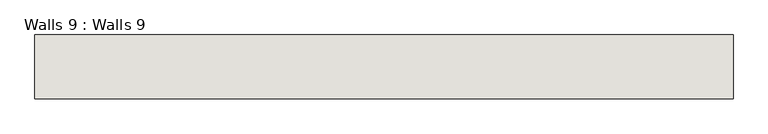
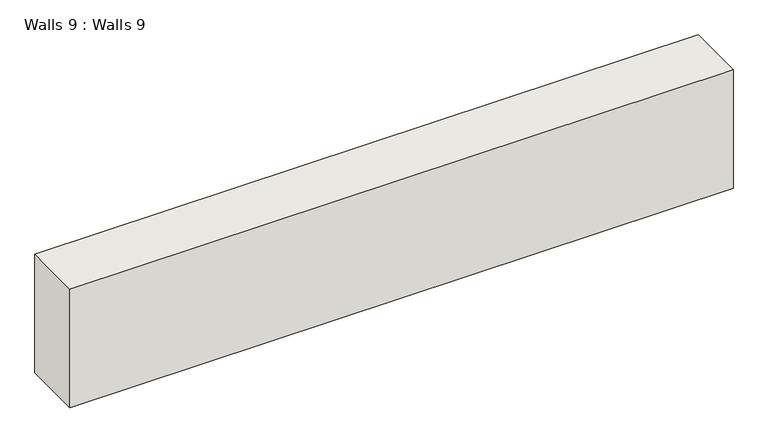
"""IFC4 building model written with IfcOpenShell, lengths in millimetres: wall geometry, Walls 9 : Walls 9."""

from ifc_helpers import new_model, si_unit, origin, origin_with_axes, place, context, project, spatial, polyline, outline, extrude, source, transform, mapped, element, save


def walls_9_walls_9_94da1e13(model_context):
    return source(origin(), model_context, "Body", "SweptSolid", [
        extrude(outline(polyline([(-9187.2996792, -7894.8501996), (-12513.0996792, -7894.8501996), (-12513.0996792, -7590.0501996), (-9187.2996792, -7590.0501996), (-9187.2996792, -7894.8501996)])), origin_with_axes(), (0.0, 0.0, 1.0), 627.4738057),
    ])


if __name__ == "__main__":
    model = new_model("IFC4")
    model_context = context("Model", 3, world=origin())
    ifc_project = project(units=[si_unit("LENGTHUNIT", "METRE", prefix="MILLI")], contexts=[model_context])
    site = spatial("IfcSite", under=ifc_project)
    building = spatial("IfcBuilding", under=site)
    placement = place(None, origin())
    walls_9_walls_9_shape = walls_9_walls_9_94da1e13(model_context)
    element("IfcWall", 1, ObjectType="Walls 9 : Walls 9", at=placement, inside=building, context=model_context, shape_type="MappedRepresentation", body=[
        mapped(walls_9_walls_9_shape, transform((0.0, 0.0, 0.0), x_axis=(1.0, 0.0, 0.0), y_axis=(0.0, 1.0, 0.0), z_axis=(0.0, 0.0, 1.0))),
    ])
    save(model, "model.ifc")

# Revit data of these elements
# Element 1 (IfcWall, "Walls 9 : Walls 9")
#   Materials on its faces: "Default Wall"
# Materials
#   "Default Wall": colour RGB 80 80 80, transparency 0
